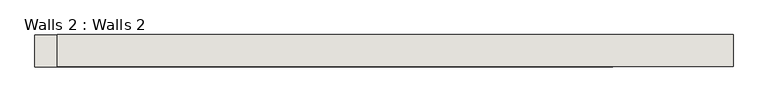
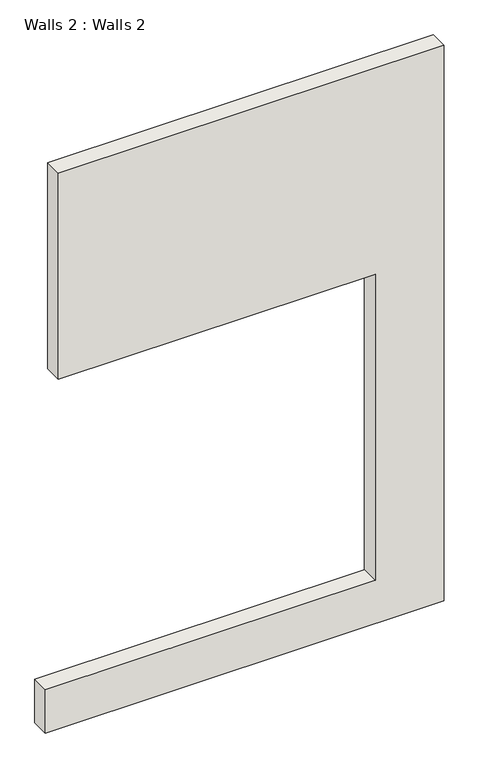
"""IFC4 building model written with IfcOpenShell, lengths in millimetres: wall geometry, Walls 2 : Walls 2."""

from ifc_helpers import new_model, si_unit, frame, origin, place, context, project, spatial, polyline, outline, extrude, source, transform, mapped, element, save


def walls_2_walls_2_432dc62d(model_context):
    return source(origin(), model_context, "Body", "SweptSolid", [
        extrude(outline(polyline([(10613.3230912, -7773.0932708), (10613.3230912, -12345.0932708), (8036.6146246, -12345.0932708), (8036.6146246, -8588.6866754), (4200.8502631, -8588.6866754), (4200.8502631, -12497.8429449), (3657.6, -12497.8429449), (3657.6, -7773.0932708), (4222.2567089, -7773.0932708), (8036.6146246, -7773.0932708), (10613.3230912, -7773.0932708)])), frame((0.0, 245.0399767, 0.0), z_axis=(0.0, 1.0, 0.0), x_axis=(0.0, 0.0, 1.0)), (0.0, 0.0, 1.0), 217.0305568),
    ])


if __name__ == "__main__":
    model = new_model("IFC4")
    model_context = context("Model", 3, world=origin())
    ifc_project = project(units=[si_unit("LENGTHUNIT", "METRE", prefix="MILLI")], contexts=[model_context])
    site = spatial("IfcSite", under=ifc_project)
    building = spatial("IfcBuilding", under=site)
    placement = place(None, origin())
    walls_2_walls_2_shape = walls_2_walls_2_432dc62d(model_context)
    element("IfcWall", 1, ObjectType="Walls 2 : Walls 2", at=placement, inside=building, context=model_context, shape_type="MappedRepresentation", body=[
        mapped(walls_2_walls_2_shape, transform((0.0, 0.0, 0.0), x_axis=(1.0, 0.0, 0.0), y_axis=(0.0, 1.0, 0.0), z_axis=(0.0, 0.0, 1.0))),
    ])
    save(model, "model.ifc")

# Revit data of these elements
# Element 1 (IfcWall, "Walls 2 : Walls 2")
#   Materials on its faces: "Default Wall"
# Materials
#   "Default Wall": colour RGB 128 128 128, transparency 0
